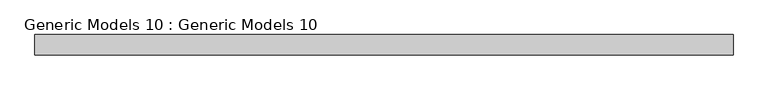
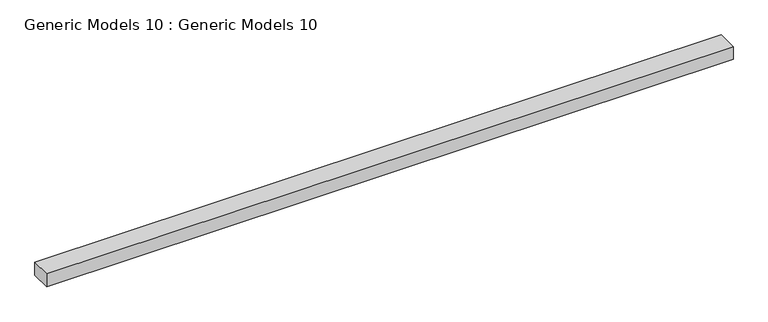
"""IFC4 building model written with IfcOpenShell, lengths in millimetres: proxy geometry, Generic Models 10 : Generic Models 10."""

from ifc_helpers import new_model, si_unit, frame, origin, place, context, project, spatial, polyline, outline, extrude, source, transform, mapped, element, save


def generic_models_10_generic_models_10_e252aed2(model_context):
    return source(origin(), model_context, "Body", "SweptSolid", [
        extrude(outline(polyline([(370.9413992, -7793.0478449), (-4797.9586008, -7793.0478449), (-4797.9586008, -7640.6478449), (370.9413992, -7640.6478449), (370.9413992, -7793.0478449)])), frame((0.0, 0.0, 6400.8), z_axis=(0.0, 0.0, 1.0), x_axis=(1.0, 0.0, 0.0)), (0.0, 0.0, 1.0), 101.6),
    ])


if __name__ == "__main__":
    model = new_model("IFC4")
    model_context = context("Model", 3, world=origin())
    ifc_project = project(units=[si_unit("LENGTHUNIT", "METRE", prefix="MILLI")], contexts=[model_context])
    site = spatial("IfcSite", under=ifc_project)
    building = spatial("IfcBuilding", under=site)
    placement = place(None, origin())
    generic_models_10_generic_models_10_shape = generic_models_10_generic_models_10_e252aed2(model_context)
    element("IfcBuildingElementProxy", 1, Name="Generic Models 10 : Generic Models 10", ObjectType="Generic Models 10 : Generic Models 10", at=placement, inside=building, context=model_context, shape_type="MappedRepresentation", body=[
        mapped(generic_models_10_generic_models_10_shape, transform((0.0, 0.0, 0.0), x_axis=(1.0, 0.0, 0.0), y_axis=(0.0, 1.0, 0.0), z_axis=(0.0, 0.0, 1.0))),
    ])
    save(model, "model.ifc")

# Revit data of these elements
# Element 1 (IfcBuildingElementProxy, "Generic Models 10 : Generic Models 10")
#   Materials on its faces: "Clad - White"
# Materials
#   "Clad - White": class "Wood", colour RGB 242 242 238, transparency 0, Cost = 0
